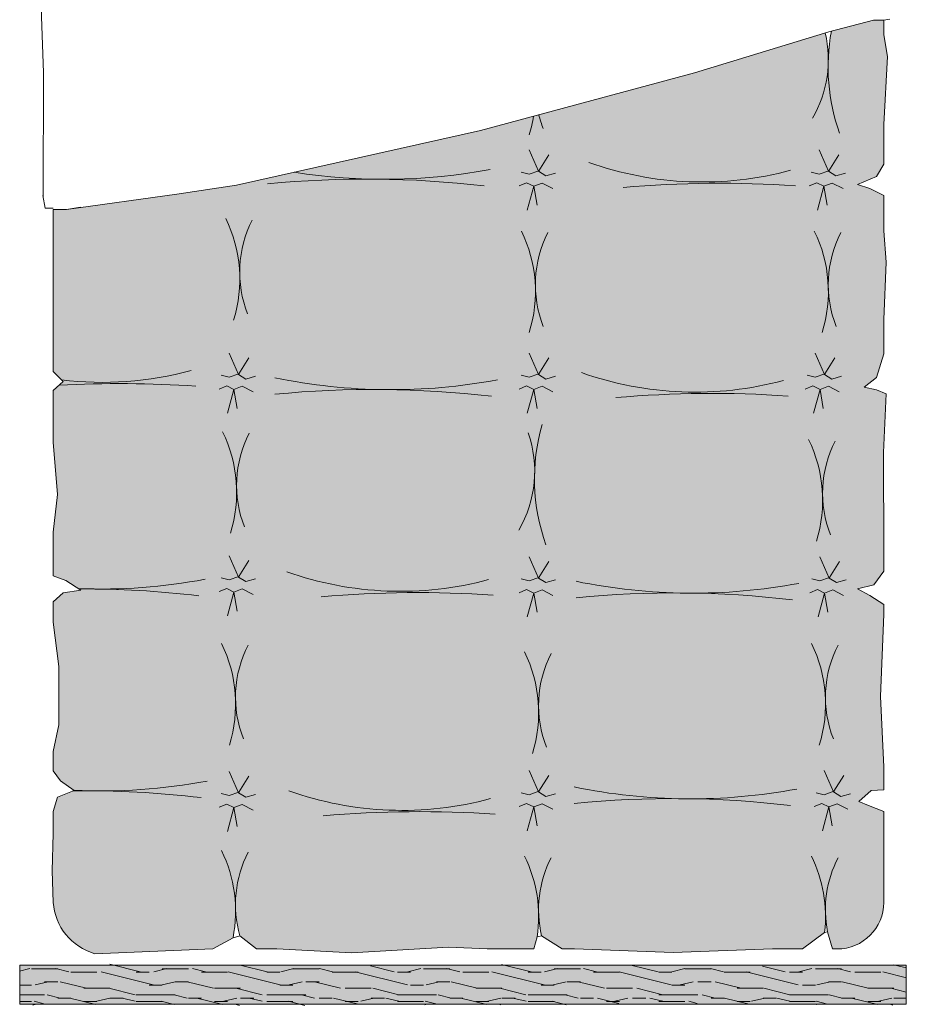
# Model space of a CAD drawing. Units: inches. Extents: x 1994 to 3075, y 3517 to 3950.
# Tile 18 of 58: x 1994.71013 to 1994.74753, y 3553.235 to 3553.27657. Entities that reach past the tile are written whole.
import ezdxf

# ---------------------------------------------------------------- set-up
doc = ezdxf.new("R2010")
doc.units = ezdxf.units.IN
doc.layers.add('A-FURN-REFR', color=8, linetype='Continuous', lineweight=13)
doc.layers.add('A-FURN-REFR-PATT', color=8, linetype='Continuous', lineweight=13)

msp = doc.modelspace()

# ---------------------------------------------------------------- hatches: boundary and pattern name
at = {"layer": 'A-FURN-REFR-PATT'}
h = msp.add_hatch(color=256, dxfattribs=at)
h.set_gradient(color1=(238, 215, 180), color2=(243, 226, 201), one_color=1, tint=0.8700000047683715)
edge = h.paths.add_edge_path()
edge.add_line((1994.745465238979, 3553.252543770607), (1994.745983417828, 3553.25225612802))
edge.add_line((1994.745983417828, 3553.25225612802), (1994.746580376501, 3553.251881311399))
edge.add_line((1994.746580376501, 3553.251881311399), (1994.746580376501, 3553.25147861202))
edge.add_line((1994.746580376501, 3553.25147861202), (1994.746444020425, 3553.247999023068))
edge.add_line((1994.746444020425, 3553.247999023068), (1994.746580376501, 3553.245035426197))
edge.add_line((1994.746580376501, 3553.245035426197), (1994.746580376501, 3553.244057442249))
edge.add_line((1994.746580376501, 3553.244057442249), (1994.746040993021, 3553.244029560099))
edge.add_line((1994.74604099302, 3553.244029560098), (1994.745522814171, 3553.24356933293))
edge.add_line((1994.745522814171, 3553.24356933293), (1994.745925842637, 3553.243396747134))
edge.add_line((1994.745925842637, 3553.243396747134), (1994.746580376501, 3553.243136987305))
edge.add_line((1994.746580376501, 3553.243136987305), (1994.746580376501, 3553.239308473302))
edge.add_ellipse((1994.744611872564, 3553.239308473302), major_axis=(-0.0013954107568795, 0.0013884655449815), ratio=0.9999999999995969, start_angle=134.8570588413608, end_angle=224.8570588413444, ccw=False)
edge.add_line((1994.744611872564, 3553.237339969366), (1994.744419991744, 3553.237339969366))
edge.add_line((1994.744419991744, 3553.237339969366), (1994.744207350188, 3553.238064686622))
edge.add_ellipse((1994.74891501896, 3553.23899557781), major_axis=(-0.0034017353614211, 0.0033848043088335), ratio=0.9999999999961552, start_angle=46.9904168057862, end_angle=56.04239135558288, ccw=False)
edge.add_ellipse((1994.738320716176, 3553.238701604092), major_axis=(0.0040909414474347, 0.0041114046525301), ratio=0.9999999999404371, start_angle=315.9964899997492, end_angle=316.8965310452939)
edge.add_ellipse((1994.74891501896, 3553.23899557781), major_axis=(-0.0034017353615801, 0.0033848043089917), ratio=0.999999999999969, start_angle=45.90260423888249, end_angle=46.99041680598647)
edge.add_ellipse((1994.738320716176, 3553.238701604092), major_axis=(-0.0041114046547348, 0.0040909414496284), ratio=0.9999999999992981, start_angle=218.3076497279251, end_angle=225.9964899996222, ccw=False)
edge.add_line((1994.744082817506, 3553.238040061614), (1994.743146211789, 3553.237339969366))
edge.add_line((1994.743146211789, 3553.237339969366), (1994.741879553322, 3553.237339969366))
edge.add_line((1994.741879553322, 3553.237339969366), (1994.737692562603, 3553.237183674896))
edge.add_line((1994.737692562603, 3553.237183674896), (1994.733531122905, 3553.237339969366))
edge.add_line((1994.733531122905, 3553.237339969366), (1994.733012944056, 3553.237339969366))
edge.add_line((1994.733012944056, 3553.237339969366), (1994.732142059715, 3553.237890147645))
edge.add_ellipse((1994.736811524591, 3553.238996855125), major_axis=(0.003384804308798, 0.0034017353613854), ratio=0.9999999999991601, start_angle=136.9904168061205, end_angle=148.1906707088415, ccw=False)
edge.add_ellipse((1994.726217221807, 3553.238702881407), major_axis=(-0.0041114046563086, 0.0040909414511943), ratio=0.9999999999589329, start_angle=225.9964899994617, end_angle=226.8965310452883)
edge.add_ellipse((1994.736811524591, 3553.238996855125), major_axis=(-0.0034017353616, 0.0033848043090115), ratio=0.9999999999992102, start_angle=45.90260423888252, end_angle=46.99041680597979)
edge.add_ellipse((1994.726217221807, 3553.238702881407), major_axis=(0.0040909414496365, 0.004111404654743), ratio=0.9999999999998221, start_angle=306.35556291123595, end_angle=315.99648999952274, ccw=False)
edge.add_line((1994.731953444552, 3553.237845444061), (1994.731817558786, 3553.237339969366))
edge.add_line((1994.731817558786, 3553.237339969366), (1994.729846297889, 3553.237339969366))
edge.add_line((1994.729846297889, 3553.237339969366), (1994.728214507854, 3553.237409828841))
edge.add_line((1994.728214507854, 3553.237409828841), (1994.724126656494, 3553.237179715257))
edge.add_line((1994.724126656494, 3553.237179715257), (1994.720979688623, 3553.237339969366))
edge.add_line((1994.720979688623, 3553.237339969366), (1994.720116058622, 3553.237339969366))
edge.add_line((1994.720116058622, 3553.237339969366), (1994.719418569442, 3553.237896439695))
edge.add_ellipse((1994.724028450143, 3553.239229745213), major_axis=(0.0033848043087955, 0.003401735361383), ratio=0.9999999999994543, start_angle=136.9904168061405, end_angle=150.9883963242237, ccw=False)
edge.add_ellipse((1994.713434147359, 3553.238935771494), major_axis=(-0.0041114046562385, 0.0040909414511246), ratio=0.9999999999586175, start_angle=225.9964899994838, end_angle=226.8965310452442)
edge.add_ellipse((1994.724028450143, 3553.239229745213), major_axis=(0.0033848043066325, 0.0034017353592091), ratio=0.9999999999427059, start_angle=135.9026042389893, end_angle=136.9904168059202)
edge.add_ellipse((1994.713434147359, 3553.238935771494), major_axis=(0.0040909414496316, 0.004111404654738), ratio=0.9999999999988398, start_angle=303.6775311936519, end_angle=315.99648999963307, ccw=False)
edge.add_line((1994.719124042928, 3553.237811254448), (1994.718273646114, 3553.237339969366))
edge.add_line((1994.718273646114, 3553.237339969366), (1994.713290858704, 3553.237138047984))
edge.add_ellipse((1994.713981582004, 3553.239489970725), major_axis=(0.0017289677196812, 0.0017376161497567), ratio=0.9999999999998783, start_angle=139.1032804179422, end_angle=208.4903617465707, ccw=False)
edge.add_line((1994.711537057931, 3553.239308473302), (1994.711495025274, 3553.240641762328))
edge.add_line((1994.711495025274, 3553.240641762328), (1994.711537057931, 3553.242218732161))
edge.add_line((1994.711537057931, 3553.242218732161), (1994.711537057931, 3553.243139187105))
edge.add_line((1994.711537057931, 3553.243139187105), (1994.711725327103, 3553.243748298751))
edge.add_line((1994.711725327103, 3553.243748298751), (1994.712371387265, 3553.244017270866))
edge.add_ellipse((1994.712804930991, 3553.201258781263), major_axis=(-0.030311711425235, 0.0301608445512322), ratio=0.9999999999998488, start_angle=314.7424189967481, end_angle=315.43798147785856, ccw=False)
edge.add_ellipse((1994.713561032044, 3553.268365279359), major_axis=(0.017178658539876, 0.0172645875167344), ratio=0.9999999999995717, start_angle=223.2793960877664, end_angle=225.1436524008468)
edge.add_ellipse((1994.712804930991, 3553.201258781263), major_axis=(0.0301608445493612, 0.0303117114233546), ratio=0.9999999999998355, start_angle=43.68062949186479, end_angle=44.7424189967496)
edge.add_ellipse((1994.713561032044, 3553.268365279359), major_axis=(-0.0172645875178435, 0.0171786585409796), ratio=0.99999999999105, start_angle=132.1588264661551, end_angle=133.2793960877638, ccw=False)
edge.add_line((1994.712414498921, 3553.244037152568), (1994.711840477486, 3553.244438640111))
edge.add_line((1994.711840477486, 3553.244438640111), (1994.71153705793, 3553.244865040809))
edge.add_line((1994.711537057931, 3553.244865040809), (1994.711537057931, 3553.24567043896))
edge.add_line((1994.711537057931, 3553.24567043896), (1994.711782902294, 3553.246797306171))
edge.add_line((1994.711782902294, 3553.246797306171), (1994.711782902294, 3553.24927102963))
edge.add_line((1994.711782902294, 3553.24927102963), (1994.711537057931, 3553.251135641442))
edge.add_line((1994.711537057931, 3553.251135641442), (1994.711537057931, 3553.25199856799))
edge.add_line((1994.711537057931, 3553.25199856799), (1994.71195562787, 3553.252377566053))
edge.add_line((1994.71195562787, 3553.252377566053), (1994.712704108549, 3553.252492622845))
edge.add_line((1994.712704108549, 3553.252492622845), (1994.712627747323, 3553.252541176693))
edge.add_ellipse((1994.712711338535, 3553.209780570924), major_axis=(-0.0303117114363433, 0.0301608445622852), ratio=0.999999999993631, start_angle=314.74241899675263, end_angle=314.96906421360694, ccw=False)
edge.add_ellipse((1994.713467439589, 3553.27688706902), major_axis=(0.017178658539876, 0.0172645875167344), ratio=0.9999999999995717, start_angle=223.2793960877664, end_angle=225.1436524008468)
edge.add_ellipse((1994.712711338535, 3553.209780570924), major_axis=(0.0301608445493616, 0.030311711423355), ratio=0.9999999999998095, start_angle=43.68062949186329, end_angle=44.7424189967481)
edge.add_ellipse((1994.713467439589, 3553.27688706902), major_axis=(-0.0172645875254605, 0.0171786585485587), ratio=0.9999999999355926, start_angle=132.8607499557009, end_angle=133.279396087769, ccw=False)
edge.add_line((1994.712619025911, 3553.252546722153), (1994.712070779315, 3553.252895321616))
edge.add_line((1994.712070779315, 3553.252895321616), (1994.71153705793, 3553.25309160873))
edge.add_line((1994.711537057931, 3553.25309160873), (1994.711537057931, 3553.254932519226))
edge.add_line((1994.711537057931, 3553.254932519225), (1994.711725327103, 3553.256519614211))
edge.add_line((1994.711725327103, 3553.256519614212), (1994.711537057931, 3553.258729396401))
edge.add_line((1994.711537057931, 3553.258729396401), (1994.711537057931, 3553.26091547788))
edge.add_line((1994.711537057931, 3553.26091547788), (1994.71195562787, 3553.261294475334))
edge.add_line((1994.71195562787, 3553.261294475334), (1994.71153705793, 3553.261720876032))
edge.add_line((1994.711537057931, 3553.261720876032), (1994.711537057931, 3553.268553942703))
edge.add_line((1994.711537057931, 3553.268553942703), (1994.712094041614, 3553.268553942703))
edge.add_line((1994.712094041614, 3553.268553942703), (1994.71674814572, 3553.269206179745))
edge.add_line((1994.71674814572, 3553.269206179745), (1994.719275959651, 3553.269584475613))
edge.add_line((1994.719275959651, 3553.269584475613), (1994.721704827398, 3553.270129843608))
edge.add_ellipse((1994.725499537882, 3553.294187533932), major_axis=(-0.0172645875167904, 0.0171786585399318), ratio=0.999999999999914, start_angle=125.8934301562025, end_angle=135.1436524012626)
edge.add_ellipse((1994.724743436827, 3553.227081035835), major_axis=(-0.0303117114243903, 0.0301608445503917), ratio=0.9999999999981067, start_angle=-46.31937050837215, end_angle=-45.257581003015)
edge.add_ellipse((1994.725499537882, 3553.294187533932), major_axis=(0.0171786585399121, 0.0172645875167707), ratio=0.9999999999996129, start_angle=215.8934301562025, end_angle=223.2793960873529, ccw=False)
edge.add_line((1994.721704827398, 3553.270129843608), (1994.729568916782, 3553.271895613963))
edge.add_line((1994.729568916782, 3553.271895613963), (1994.738589710934, 3553.274322309254))
edge.add_line((1994.738589710934, 3553.274322309254), (1994.744109518087, 3553.276010668554))
edge.add_ellipse((1994.739263851125, 3553.274892925541), major_axis=(0.0035075950851018, 0.0035251403466364), ratio=0.9999999999978005, start_angle=315.5146379508602, end_angle=327.8461990640952, ccw=False)
edge.add_ellipse((1994.752502542269, 3553.27457735018), major_axis=(-0.005865536420184, 0.0058363425837936), ratio=0.999999999997771, start_angle=42.27583207499214, end_angle=44.70724330108613)
edge.add_ellipse((1994.739263851125, 3553.274892925541), major_axis=(-0.0035251403464673, 0.0035075950849335), ratio=0.9999999999932054, start_angle=221.46843742522, end_angle=225.5146379508603)
edge.add_ellipse((1994.752502542269, 3553.27457735018), major_axis=(0.0058363425838986, 0.0058655364202896), ratio=0.9999999999968727, start_angle=124.36393844595369, end_angle=132.2758320749922, ccw=False)
edge.add_line((1994.744366414854, 3553.276084281811), (1994.746144687441, 3553.276547800884))
edge.add_line((1994.746144687441, 3553.276547800884), (1994.746580376501, 3553.276547800884))
edge.add_line((1994.746580376501, 3553.276547800884), (1994.746580376501, 3553.275937280929))
edge.add_line((1994.746580376501, 3553.275937280929), (1994.746736751779, 3553.275017923455))
edge.add_line((1994.746736751779, 3553.275017923455), (1994.7465803765, 3553.272140403147))
edge.add_line((1994.746580376501, 3553.272140403147), (1994.746580376501, 3553.270472078447))
edge.add_line((1994.746580376501, 3553.270472078447), (1994.746276149182, 3553.269955419744))
edge.add_line((1994.746276149182, 3553.269955419744), (1994.745470093312, 3553.269610249368))
edge.add_line((1994.745470093312, 3553.269610249368), (1994.745988272162, 3553.269437663573))
edge.add_line((1994.745988272162, 3553.269437663573), (1994.7465803765, 3553.269148924124))
edge.add_line((1994.746580376501, 3553.269148924124), (1994.746580376501, 3553.267653184612))
edge.add_line((1994.746580376501, 3553.267653184612), (1994.746679176587, 3553.266331127757))
edge.add_line((1994.746679176587, 3553.266331127757), (1994.7465803765, 3553.263913835225))
edge.add_line((1994.746580376501, 3553.263913835225), (1994.746580376501, 3553.262466545988))
edge.add_line((1994.746580376501, 3553.262466545988), (1994.746271294849, 3553.261460679889))
edge.add_line((1994.746271294849, 3553.261460679889), (1994.745753115999, 3553.261057981117))
edge.add_line((1994.745753115999, 3553.261057981117), (1994.746271294849, 3553.260942923717))
edge.add_line((1994.746271294849, 3553.260942923717), (1994.746674322254, 3553.260770338529))
edge.add_line((1994.746674322254, 3553.260770338529), (1994.74655917187, 3553.258296615677))
edge.add_line((1994.74655917187, 3553.258296615677), (1994.746580376501, 3553.25406739227))
edge.add_line((1994.746580376501, 3553.25406739227), (1994.746580376501, 3553.253291640363))
edge.add_line((1994.746580376501, 3553.253291640363), (1994.746156143405, 3553.252716355795))
edge.add_line((1994.746156143405, 3553.252716355795), (1994.745465238979, 3553.252543770607))
edge = h.paths.add_edge_path(flags=16)
edge.add_ellipse((1994.737756386553, 3553.209608254897), major_axis=(0.030160844549362, 0.0303117114233554), ratio=0.9999999999997834, start_angle=43.68062949186179, end_angle=44.74241899674661)
edge.add_ellipse((1994.738512487607, 3553.276714752993), major_axis=(0.0171786585398764, 0.0172645875167348), ratio=0.9999999999995255, start_angle=223.2793960877637, end_angle=225.1436524008441)
edge = h.paths.add_edge_path(flags=16)
edge.add_ellipse((1994.72687704885, 3553.257511810059), major_axis=(-0.0035251403466965, 0.0035075950851616), ratio=0.9999999999998879, start_angle=221.4684374256727, end_angle=225.514637950396)
edge.add_ellipse((1994.740115739994, 3553.257196234698), major_axis=(0.0058363425840069, 0.0058655364203984), ratio=0.9999999999987389, start_angle=132.2758320752676, end_angle=134.7072433008111)
h.paths.add_polyline_path([(1994.732021808397, 3553.253023267114), (1994.731986786092, 3553.253010769348), (1994.73200619594, 3553.252998522719)], flags=16)
edge = h.paths.add_edge_path(flags=16)
edge.add_ellipse((1994.726217221807, 3553.247322021218), major_axis=(0.0040909414477731, 0.0041114046528702), ratio=0.9999999999458513, start_angle=315.9964899995724, end_angle=316.8965310452884)
edge.add_ellipse((1994.736811524591, 3553.247615994937), major_axis=(-0.0034017353615801, 0.0033848043089917), ratio=0.999999999999969, start_angle=45.90260423888249, end_angle=46.99041680598647)
h.paths.add_polyline_path([(1994.73200619594, 3553.261594210102), (1994.732021808397, 3553.261618954497), (1994.731986786092, 3553.261606456731)], flags=16)
edge = h.paths.add_edge_path(flags=16)
edge.add_ellipse((1994.748793777434, 3553.256584102472), major_axis=(-0.0034017353616, 0.0033848043090115), ratio=0.9999999999992102, start_angle=45.90260423888252, end_angle=46.99041680597979)
edge.add_ellipse((1994.73819947465, 3553.256290128754), major_axis=(0.0040909414477996, 0.0041114046528968), ratio=0.9999999999466499, start_angle=315.996489999578, end_angle=316.8965310452884)
h.paths.add_polyline_path([(1994.744250725601, 3553.253010769348), (1994.744270135448, 3553.252998522719), (1994.744285747906, 3553.253023267114)], flags=16)
edge = h.paths.add_edge_path(flags=16)
edge.add_ellipse((1994.725807702035, 3553.285306483294), major_axis=(0.0171786585398506, 0.0172645875167089), ratio=0.9999999999995244, start_angle=223.279396087769, end_angle=225.1436524008441)
edge.add_ellipse((1994.725051600982, 3553.218199985198), major_axis=(0.0301608445493262, 0.0303117114233194), ratio=0.9999999999998141, start_angle=43.68062949186629, end_angle=44.74241899674811)
edge = h.paths.add_edge_path(flags=16)
edge.add_ellipse((1994.74891501896, 3553.247973753577), major_axis=(-0.0034017353616, 0.0033848043090115), ratio=0.9999999999992102, start_angle=45.90260423888252, end_angle=46.99041680597979)
edge.add_ellipse((1994.738320716176, 3553.247679779859), major_axis=(0.0040909414477996, 0.0041114046528968), ratio=0.9999999999466499, start_angle=315.996489999578, end_angle=316.8965310452884)
edge = h.paths.add_edge_path(flags=16)
edge.add_ellipse((1994.726082432568, 3553.265091023611), major_axis=(0.0040909414477996, 0.0041114046528968), ratio=0.9999999999466499, start_angle=315.996489999578, end_angle=316.8965310452884)
edge.add_ellipse((1994.736676735351, 3553.26538499733), major_axis=(-0.0034017353616, 0.0033848043090115), ratio=0.9999999999992102, start_angle=45.90260423888252, end_angle=46.99041680597979)
h.paths.add_polyline_path([(1994.74405918212, 3553.261606456731), (1994.744078591968, 3553.261594210102), (1994.744094204425, 3553.261618954497)], flags=16)
edge = h.paths.add_edge_path(flags=16)
edge.add_ellipse((1994.749034005182, 3553.26538499733), major_axis=(-0.0034017353615801, 0.0033848043089917), ratio=0.999999999999969, start_angle=45.90260423888249, end_angle=46.99041680598647)
edge.add_ellipse((1994.738439702398, 3553.265091023611), major_axis=(0.0040909414477724, 0.0041114046528695), ratio=0.9999999999457356, start_angle=315.9964899995779, end_angle=316.896531045294)
h.paths.add_polyline_path([(1994.732021808397, 3553.243996435937), (1994.731986786092, 3553.24398393817), (1994.73200619594, 3553.243971691542)], flags=16)
edge = h.paths.add_edge_path(flags=16)
edge.add_ellipse((1994.737679105019, 3553.20092495741), major_axis=(0.0301608445494179, 0.0303117114234116), ratio=0.9999999999999388, start_angle=43.68062949186479, end_angle=44.74241899675109)
edge.add_ellipse((1994.738435206073, 3553.268031455506), major_axis=(0.0171786585398771, 0.0172645875167355), ratio=0.9999999999995772, start_angle=223.2793960877664, end_angle=225.1436524008493)
h.paths.add_polyline_path([(1994.744468735191, 3553.243996435937), (1994.744433712885, 3553.24398393817), (1994.744453122734, 3553.243971691542)], flags=16)
h.paths.add_polyline_path([(1994.73200619594, 3553.270171481), (1994.732021808397, 3553.270196225395), (1994.731986786092, 3553.270183727629)], flags=16)
h.paths.add_polyline_path([(1994.719369026331, 3553.253065718053), (1994.719334004026, 3553.253053220288), (1994.719353413874, 3553.253040973658)], flags=16)
edge = h.paths.add_edge_path(flags=16)
edge.add_ellipse((1994.713477879544, 3553.256619851287), major_axis=(-0.0041114046560738, 0.0040909414509607), ratio=0.999999999962278, start_angle=225.9964899995778, end_angle=226.8965310452884)
edge.add_ellipse((1994.724072182329, 3553.256913825005), major_axis=(0.0033848043069108, 0.0034017353594889), ratio=0.9999999999478042, start_angle=135.9026042388825, end_angle=136.9904168059803)
h.paths.add_polyline_path([(1994.744223325676, 3553.270183727629), (1994.744242735524, 3553.270171481), (1994.744258347981, 3553.270196225395)], flags=16)
edge = h.paths.add_edge_path(flags=16)
edge.add_ellipse((1994.713434147359, 3553.247679779859), major_axis=(0.004090941447773, 0.0041114046528701), ratio=0.999999999945836, start_angle=315.9964899995722, end_angle=316.896531045288)
edge.add_ellipse((1994.724028450143, 3553.247973753577), major_axis=(-0.0034017353616392, 0.0033848043090505), ratio=0.999999999998303, start_angle=45.9026042388825, end_angle=46.99041680598649)
h.paths.add_polyline_path([(1994.719353413874, 3553.261594210102), (1994.719369026331, 3553.261618954497), (1994.719334004026, 3553.261606456731)], flags=16)
edge = h.paths.add_edge_path(flags=16)
edge.add_ellipse((1994.713610336299, 3553.265618953796), major_axis=(-0.0041114046594229, 0.0040909414542932), ratio=0.9999999998956695, start_angle=225.9964899995777, end_angle=226.896531045288)
edge.add_ellipse((1994.724204639084, 3553.265912927514), major_axis=(-0.0034017353616, 0.0033848043090115), ratio=0.9999999999992102, start_angle=45.90260423888252, end_angle=46.99041680597979)
h.paths.add_polyline_path([(1994.719369026331, 3553.243962374809), (1994.719334004026, 3553.243949877043), (1994.719353413874, 3553.243937630414)], flags=16)
msp.add_hatch(color=256, dxfattribs=at).paths.add_polyline_path([(1994.74752711248, 3553.236652102432), (1994.710125537677, 3553.236652102432), (1994.710125537677, 3553.235003554395), (1994.74752711248, 3553.235003554395)])
h = msp.add_hatch(dxfattribs=at)
h.set_pattern_fill('LEGNO1', color=256, scale=0.005511811023622, style=0, pattern_type=2)
h.set_pattern_definition([(0, (2000.356371596277, 3548.843453761226), (0, 0.005511811023622), [0.0011023622047244, -0.0016535433070866, 0.0005511811023622, -0.0022047244094488]), (0, (2000.360229863994, 3548.843591556501), (0, 0.005511811023622), [0.0011023622047244, -0.0044094488188976]), (0, (2000.359678682892, 3548.843867147053), (0, 0.005511811023622), [0.0005511811023622, -0.0049606299212598]), (0, (2000.356647186829, 3548.844004942328), (0, 0.005511811023622), [0.0002755905511811, -0.0038582677165354, 0.0002755905511811, -0.0011023622047244]), (0, (2000.358576320687, 3548.844280532879), (0, 0.005511811023622), [0.0011023622047244, -0.0016535433070866, 0.0002755905511811, -0.0024803149606299]), (0, (2000.357198367931, 3548.844418328155), (0, 0.005511811023622), [0.0008267716535433, -0.0046850393700787]), (0, (2000.358576320687, 3548.844556123431), (0, 0.005511811023622), [0.0016535433070866, -0.0038582677165354]), (0, (2000.356922777379, 3548.844693918706), (0, 0.005511811023622), [0.0011023622047244, -0.0044094488188976]), (0, (2000.35912750179, 3548.844831713982), (0, 0.005511811023622), [0.002755905511811, -0.002755905511811]), (0, (2000.357473958482, 3548.845107304533), (0, 0.005511811023622), [0.0005511811023622, -0.0016535433070866, 0.0011023622047244, -0.0022047244094488]), (0, (2000.361332226199, 3548.845245099808), (0, 0.005511811023622), [0.0011023622047244, -0.0044094488188976]), (0, (2000.360229863994, 3548.845382895084), (0, 0.005511811023622), [0.0005511811023622, -0.0049606299212598]), (0, (2000.35912750179, 3548.84552069036), (0, 0.005511811023622), [0.0005511811023622, -0.0049606299212598]), (0, (2000.356371596277, 3548.845658485635), (0, 0.005511811023622), [0.0011023622047244, -0.0044094488188976]), (0, (2000.35912750179, 3548.845796280911), (0, 0.005511811023622), [0.0011023622047244, -0.0044094488188976]), (0, (2000.35912750179, 3548.846071871462), (0, 0.005511811023622), [0.0011023622047244, -0.0011023622047244, 0.0011023622047244, -0.0022047244094488]), (0, (2000.358025139584, 3548.846347462013), (0, 0.005511811023622), [0.0005511811023622, -0.002755905511811, 0.0011023622047244, -0.0011023622047244]), (0, (2000.35912750179, 3548.846485257289), (0, 0.005511811023622), [0.0016535433070866, -0.0038582677165354]), (0, (2000.35912750179, 3548.84676084784), (0, 0.005511811023622), [0.0011023622047244, -0.0044094488188976]), (0, (2000.356922777379, 3548.846898643116), (0, 0.005511811023622), [0.0016535433070866, -0.0022047244094488, 0.0005511811023622, -0.0011023622047244]), (0, (2000.356922777379, 3548.847174233667), (0, 0.005511811023622), [0.002755905511811, -0.002755905511811]), (0, (2000.360229863994, 3548.847312028942), (0, 0.005511811023622), [0.0005511811023622, -0.0049606299212598]), (0, (2000.358576320687, 3548.847449824219), (0, 0.005511811023622), [0.0011023622047244, -0.0044094488188976]), (0, (2000.357473958482, 3548.847587619493), (0, 0.005511811023622), [0.0005511811023622, -0.0022047244094488, 0.0005511811023622, -0.0022047244094488]), (0, (2000.356922777379, 3548.84772541477), (0, 0.005511811023622), [0.0005511811023622, -0.0016535433070866, 0.0011023622047244, -0.0022047244094488]), (0, (2000.358025139584, 3548.847863210045), (0, 0.005511811023622), [0.0005511811023622, -0.002755905511811, 0.0005511811023622, -0.0016535433070866]), (0, (2000.35912750179, 3548.84800100532), (0, 0.005511811023622), [0.0016535433070866, -0.0038582677165354]), (0, (2000.356922777379, 3548.848276595871), (0, 0.005511811023622), [0.0011023622047244, -0.0044094488188976]), (0, (2000.359678682892, 3548.848414391147), (0, 0.005511811023622), [0.0005511811023622, -0.0049606299212598]), (0, (2000.360781045096, 3548.848552186423), (0, 0.005511811023622), [0.0005511811023622, -0.0049606299212598]), (14.03624347, (2000.360229863994, 3548.843867147053), (0.0055118110234648, -2.016e-13), [0.0005677165354331, -0.0221580619543307]), (14.03624347, (2000.360781045096, 3548.845107304533), (0.0055118110234648, -2.016e-13), [0.0005677165354331, -0.0221580619543307]), (14.03624347, (2000.360229863994, 3548.848414391147), (0.0055118110234648, -2.016e-13), [0.0005677165354331, -0.0221580619543307]), (14.03624347, (2000.358576320687, 3548.846347462013), (0.0055118110234648, -2.016e-13), [0.0005677165354331, -0.0221580619543307]), (14.03624347, (2000.359678682892, 3548.847174233667), (0.0055118110234648, -2.016e-13), [0.0005677165354331, -0.0221580619543307]), (14.03624347, (2000.360229863994, 3548.84676084784), (0.0055118110234648, -2.016e-13), [0.0005677165354331, -0.0221580619543307]), (14.03624347, (2000.357473958482, 3548.84772541477), (0.0055118110234648, -2.016e-13), [0.0005677165354331, -0.0221580619543307]), (14.03624347, (2000.359678682892, 3548.847449824219), (0.0055118110234648, -2.016e-13), [0.0005677165354331, -0.0221580619543307]), (14.03624347, (2000.360781045096, 3548.845382895084), (0.0055118110234648, -2.016e-13), [0.0011354330708661, -0.0215903454188977]), (14.03624347, (2000.360229863994, 3548.845796280911), (0.0055118110234648, -2.016e-13), [0.0011354330708661, -0.0215903454188977]), (14.03624347, (2000.360229863994, 3548.846071871462), (0.0055118110234648, -2.016e-13), [0.0011354330708661, -0.0215903454188977]), (165.96375653, (2000.358576320687, 3548.844280532879), (-0.0055118110234648, -2.016e-13), [0.0005677165354331, -0.0011354330708661, 0.0005677165354331, -0.0204549123480315]), (165.96375653, (2000.357473958482, 3548.845107304533), (-0.0055118110234648, -2.016e-13), [0.0005677165354331, -0.0221580619543307]), (165.96375653, (2000.357473958482, 3548.847587619493), (-0.0055118110234648, -2.016e-13), [0.0011354330708661, -0.0215903454188977]), (194.03624347, (2000.360229863994, 3548.843591556501), (-0.0055118110234648, 2.016e-13), [0.0005677165354331, -0.0221580619543307]), (345.96375653, (2000.361332226199, 3548.843591556501), (0.0055118110234648, 2.016e-13), [0.0005677165354331, -0.0221580619543307]), (345.96375653, (2000.359678682892, 3548.84552069036), (0.0055118110234648, 2.016e-13), [0.0005677165354331, -0.0221580619543307]), (345.96375653, (2000.360781045096, 3548.846485257289), (0.0055118110234648, 2.016e-13), [0.0005677165354331, -0.0221580619543307]), (345.96375653, (2000.358576320687, 3548.846898643116), (0.0055118110234648, 2.016e-13), [0.0005677165354331, -0.0221580619543307]), (345.96375653, (2000.358025139584, 3548.847587619493), (0.0055118110234648, 2.016e-13), [0.0005677165354331, -0.0221580619543307]), (345.96375653, (2000.358576320687, 3548.847863210045), (0.0055118110234648, 2.016e-13), [0.0005677165354331, -0.0221580619543307]), (345.96375653, (2000.358576320687, 3548.846898643116), (0.0055118110234648, 2.016e-13), [0.0005677165354331, -0.0221580619543307]), (345.96375653, (2000.360229863994, 3548.84772541477), (0.0055118110234648, 2.016e-13), [0.0022708661417323, -0.0204549123480315]), (345.96375653, (2000.356922777379, 3548.844004942328), (0.0055118110234648, 2.016e-13), [0.0022708661417323, -0.0204549123480315]), (345.96375653, (2000.357473958482, 3548.844418328155), (0.0055118110234648, 2.016e-13), [0.0022708661417323, -0.0204549123480315]), (345.96375653, (2000.358025139584, 3548.844693918706), (0.0055118110234648, 2.016e-13), [0.0005677165354331, -0.0011354330708661, 0.0011354330708661, -0.0198871958125984]), (345.96375653, (2000.358025139584, 3548.845107304533), (0.0055118110234648, 2.016e-13), [0.0011354330708661, -0.0011354330708661, 0.0011354330708661, -0.0193194792771654]), (345.96375653, (2000.357473958482, 3548.845658485635), (0.0055118110234648, 2.016e-13), [0.0022708661417323, -0.0204549123480315]), (345.96375653, (2000.356922777379, 3548.846071871462), (0.0055118110234648, 2.016e-13), [0.0022708661417323, -0.0204549123480315]), (345.96375653, (2000.356922777379, 3548.846347462013), (0.0055118110234648, 2.016e-13), [0.0022708661417323, -0.0204549123480315]), (345.96375653, (2000.360781045096, 3548.84800100532), (0.0055118110234648, 2.016e-13), [0.0005677165354331, -0.0221580619543307]), (345.9637675300001, (2000.361332226199, 3548.848552186423), (0.0055118110234647, 1.0583933e-09), [0.0011354330708661, -0.0215903454188977]), (345.9637675300001, (2000.358025139584, 3548.848276595871), (0.0055118110234647, 1.0583933e-09), [0.0011354330708661, -0.0215903454188977]), (345.96375753, (2000.357473958482, 3548.843453761226), (0.0055118110234648, 9.64008e-11), [0.0022708661417323, -0.0204549123480315]), (345.96375753, (2000.360781045096, 3548.847312028942), (0.0055118110234648, 9.64008e-11), [0.0017031496062992, -0.0210226288834646]), (345.96375753, (2000.361332226199, 3548.846898643116), (0.0055118110234648, 9.64008e-11), [0.0034062992125984, -0.0193194792771654])])
h.paths.add_polyline_path([(1994.74752711248, 3553.236652102432), (1994.710125537677, 3553.236652102432), (1994.710125537677, 3553.235003554395), (1994.74752711248, 3553.235003554395)])

# ---------------------------------------------------------------- linework, layer by layer
at = {"layer": 'A-FURN-REFR'}
for p, q in [((1994.710937653731, 3553.279644278879), (1994.711129775177, 3553.274346052923)), ((1994.74425661957, 3553.276055662909), (1994.746144687441, 3553.276547800884)), ((1994.746144687441, 3553.276547800884), (1994.746580376501, 3553.276547800884)), ((1994.746580376501, 3553.276547800884), (1994.746826688549, 3553.27659207166)), ((1994.746580376501, 3553.276547800884), (1994.746580376501, 3553.275937280929)), ((1994.738589710934, 3553.274322309254), (1994.74425661957, 3553.276055662909)), ((1994.746736751779, 3553.275017923455), (1994.746580376501, 3553.275937280929)), ((1994.746580376501, 3553.272140403147), (1994.746736751779, 3553.275017923455)), ((1994.711129775177, 3553.274346052923), (1994.711113967212, 3553.269074274324)), ((1994.729568916782, 3553.271895613963), (1994.738589710934, 3553.274322309254)), ((1994.719275959651, 3553.269584475613), (1994.729568916782, 3553.271895613963)), ((1994.746580376501, 3553.272140403147), (1994.746580376501, 3553.270472078447)), ((1994.73200619594, 3553.270171481), (1994.731612882744, 3553.27107177963)), ((1994.744242735524, 3553.270171481), (1994.743849422327, 3553.27107177963)), ((1994.732021808397, 3553.270196225395), (1994.732445338485, 3553.270867483972)), ((1994.744258347981, 3553.270196225395), (1994.744681878069, 3553.270867483972)), ((1994.731612882744, 3553.270050299618), (1994.732021808397, 3553.270196225395)), ((1994.732313897828, 3553.269977336729), (1994.73200619594, 3553.270171481)), ((1994.743849422327, 3553.270050299618), (1994.744258347981, 3553.270196225395)), ((1994.744550437411, 3553.269977336729), (1994.744242735524, 3553.270171481)), ((1994.746276149182, 3553.269955419744), (1994.746580376501, 3553.270472078447)), ((1994.731276980012, 3553.270137855084), (1994.731612882744, 3553.270050299618)), ((1994.732722823482, 3553.270094077351), (1994.732313897828, 3553.269977336729)), ((1994.743513519595, 3553.270137855084), (1994.743849422327, 3553.270050299618)), ((1994.744959363065, 3553.270094077351), (1994.744550437411, 3553.269977336729)), ((1994.745470093312, 3553.269610249368), (1994.746276149182, 3553.269955419744)), ((1994.71674814572, 3553.269206179745), (1994.719275959651, 3553.269584475613)), ((1994.731189353408, 3553.269554152405), (1994.731510651707, 3553.269685485605)), ((1994.731510651707, 3553.269685485605), (1994.731817345571, 3553.269539559828)), ((1994.731817345571, 3553.269539559828), (1994.731539860574, 3553.268532672393)), ((1994.732167853489, 3553.269670893028), (1994.731817345571, 3553.269539559828)), ((1994.731817345571, 3553.269539559828), (1994.731948786228, 3553.268736968482)), ((1994.732620591692, 3553.269437411783), (1994.732167853489, 3553.269670893028)), ((1994.743425892991, 3553.269554152405), (1994.74374719129, 3553.269685485605)), ((1994.74374719129, 3553.269685485605), (1994.744053885154, 3553.269539559828)), ((1994.744053885154, 3553.269539559828), (1994.743776400158, 3553.268532672393)), ((1994.744404393072, 3553.269670893028), (1994.744053885154, 3553.269539559828)), ((1994.744053885154, 3553.269539559828), (1994.744185325811, 3553.268736968482)), ((1994.744857131275, 3553.269437411783), (1994.744404393072, 3553.269670893028)), ((1994.745988272162, 3553.269437663573), (1994.745470093312, 3553.269610249368)), ((1994.746580376501, 3553.269148924124), (1994.745988272162, 3553.269437663573)), ((1994.711098697876, 3553.269150558865), (1994.711206060319, 3553.268614183581)), ((1994.712094041614, 3553.268553942703), (1994.71674814572, 3553.269206179745)), ((1994.746580376501, 3553.269148924124), (1994.746580376501, 3553.267653184612)), ((1994.711206060319, 3553.268614183581), (1994.711537057931, 3553.268614183581)), ((1994.712094041614, 3553.268553942703), (1994.711537057931, 3553.268553942703)), ((1994.711537057931, 3553.261720876032), (1994.711537057931, 3553.268553942703)), ((1994.712094041614, 3553.268553942703), (1994.712683841166, 3553.2686600201)), ((1994.746679176587, 3553.266331127757), (1994.746580376501, 3553.267653184612)), ((1994.746580376501, 3553.263913835225), (1994.746679176587, 3553.266331127757)), ((1994.746580376501, 3553.263913835225), (1994.746580376501, 3553.262466545988)), ((1994.719353413874, 3553.261594210102), (1994.718960100677, 3553.262494508731)), ((1994.719369026331, 3553.261618954497), (1994.719792556418, 3553.262290213074)), ((1994.73200619594, 3553.261594210102), (1994.731612882744, 3553.262494508731)), ((1994.732021808397, 3553.261618954497), (1994.732445338485, 3553.262290213074)), ((1994.744078591968, 3553.261594210102), (1994.743685278772, 3553.262494508731)), ((1994.744094204425, 3553.261618954497), (1994.744517734513, 3553.262290213074)), ((1994.746271294849, 3553.261460679889), (1994.746580376501, 3553.262466545988)), ((1994.711537057931, 3553.261720876032), (1994.71195562787, 3553.261294475334)), ((1994.718624197945, 3553.261560584186), (1994.718960100677, 3553.26147302872)), ((1994.718960100677, 3553.26147302872), (1994.719369026331, 3553.261618954497)), ((1994.719661115761, 3553.261400065832), (1994.719353413874, 3553.261594210102)), ((1994.720070041415, 3553.261516806453), (1994.719661115761, 3553.261400065832)), ((1994.731276980012, 3553.261560584186), (1994.731612882744, 3553.26147302872)), ((1994.731612882744, 3553.26147302872), (1994.732021808397, 3553.261618954497)), ((1994.732313897828, 3553.261400065832), (1994.73200619594, 3553.261594210102)), ((1994.732722823482, 3553.261516806453), (1994.732313897828, 3553.261400065832)), ((1994.743349376039, 3553.261560584186), (1994.743685278772, 3553.26147302872)), ((1994.743685278772, 3553.26147302872), (1994.744094204425, 3553.261618954497)), ((1994.744386293856, 3553.261400065832), (1994.744078591968, 3553.261594210102)), ((1994.744795219509, 3553.261516806453), (1994.744386293856, 3553.261400065832)), ((1994.745753115999, 3553.261057981117), (1994.746271294849, 3553.261460679889)), ((1994.71195562787, 3553.261294475334), (1994.711537057931, 3553.26091547788)), ((1994.718536571342, 3553.260976881507), (1994.71885786964, 3553.261108214707)), ((1994.71885786964, 3553.261108214707), (1994.719164563504, 3553.26096228893)), ((1994.719515071422, 3553.261093622129), (1994.719164563504, 3553.26096228893)), ((1994.719967809625, 3553.260860140885), (1994.719515071422, 3553.261093622129)), ((1994.731189353408, 3553.260976881507), (1994.731510651707, 3553.261108214707)), ((1994.731510651707, 3553.261108214707), (1994.731817345571, 3553.26096228893)), ((1994.732167853489, 3553.261093622129), (1994.731817345571, 3553.26096228893)), ((1994.732620591692, 3553.260860140885), (1994.732167853489, 3553.261093622129)), ((1994.743261749436, 3553.260976881507), (1994.743583047734, 3553.261108214707)), ((1994.743583047734, 3553.261108214707), (1994.743889741599, 3553.26096228893)), ((1994.744240249517, 3553.261093622129), (1994.743889741599, 3553.26096228893)), ((1994.74469298772, 3553.260860140885), (1994.744240249517, 3553.261093622129)), ((1994.746271294849, 3553.260942923717), (1994.745753115999, 3553.261057981117)), ((1994.711537057931, 3553.258729396401), (1994.711537057931, 3553.26091547788)), ((1994.719164563504, 3553.26096228893), (1994.718887078508, 3553.259955401496)), ((1994.719164563504, 3553.26096228893), (1994.719296004161, 3553.260159697585)), ((1994.731817345571, 3553.26096228893), (1994.731539860574, 3553.259955401496)), ((1994.731817345571, 3553.26096228893), (1994.731948786228, 3553.260159697585)), ((1994.743889741599, 3553.26096228893), (1994.743612256602, 3553.259955401496)), ((1994.743889741599, 3553.26096228893), (1994.744021182256, 3553.260159697585)), ((1994.746674322254, 3553.260770338529), (1994.746271294849, 3553.260942923717)), ((1994.74655917187, 3553.258296615677), (1994.746674322254, 3553.260770338529)), ((1994.711537057931, 3553.258729396401), (1994.711725327103, 3553.256519614212)), ((1994.746580376501, 3553.25406739227), (1994.74655917187, 3553.258296615677)), ((1994.711725327103, 3553.256519614212), (1994.711537057931, 3553.254932519225)), ((1994.711537057931, 3553.25309160873), (1994.711537057931, 3553.254932519225)), ((1994.719353413874, 3553.253040973658), (1994.718960100677, 3553.253941272288)), ((1994.746580376501, 3553.25406739227), (1994.746580376501, 3553.253291640363)), ((1994.719369026331, 3553.253065718053), (1994.719792556418, 3553.25373697663)), ((1994.73200619594, 3553.252998522719), (1994.731612882744, 3553.253898821348)), ((1994.732021808397, 3553.253023267114), (1994.732445338485, 3553.25369452569)), ((1994.744270135448, 3553.252998522719), (1994.743876822252, 3553.253898821348)), ((1994.744285747906, 3553.253023267114), (1994.744709277993, 3553.25369452569)), ((1994.746156143405, 3553.252716355795), (1994.746580376501, 3553.253291640363)), ((1994.711537057931, 3553.25309160873), (1994.712070779315, 3553.252895321616)), ((1994.712070779315, 3553.252895321616), (1994.712704108549, 3553.252492622845)), ((1994.718624197945, 3553.253007347742), (1994.718960100677, 3553.252919792276)), ((1994.718960100677, 3553.252919792276), (1994.719369026331, 3553.253065718053)), ((1994.719661115761, 3553.252846829387), (1994.719353413874, 3553.253040973658)), ((1994.720070041415, 3553.252963570009), (1994.719661115761, 3553.252846829387)), ((1994.731276980012, 3553.252964896802), (1994.731612882744, 3553.252877341336)), ((1994.731612882744, 3553.252877341336), (1994.732021808397, 3553.253023267114)), ((1994.732313897828, 3553.252804378447), (1994.73200619594, 3553.252998522719)), ((1994.732722823482, 3553.25292111907), (1994.732313897828, 3553.252804378447)), ((1994.74354091952, 3553.252964896802), (1994.743876822252, 3553.252877341336)), ((1994.743876822252, 3553.252877341336), (1994.744285747906, 3553.253023267114)), ((1994.744577837336, 3553.252804378447), (1994.744270135448, 3553.252998522719)), ((1994.74498676299, 3553.25292111907), (1994.744577837336, 3553.252804378447)), ((1994.745465238979, 3553.252543770607), (1994.746156143405, 3553.252716355795)), ((1994.71195562787, 3553.252377566053), (1994.711537057931, 3553.25199856799)), ((1994.712704108549, 3553.252492622845), (1994.71195562787, 3553.252377566053)), ((1994.718536571342, 3553.252423645063), (1994.71885786964, 3553.252554978263)), ((1994.71885786964, 3553.252554978263), (1994.719164563504, 3553.252409052485)), ((1994.719164563504, 3553.252409052485), (1994.718887078508, 3553.251402165051)), ((1994.719515071422, 3553.252540385685), (1994.719164563504, 3553.252409052485)), ((1994.719164563504, 3553.252409052485), (1994.719296004161, 3553.251606461139)), ((1994.719967809625, 3553.252306904441), (1994.719515071422, 3553.252540385685)), ((1994.731189353408, 3553.252381194124), (1994.731510651707, 3553.252512527323)), ((1994.731510651707, 3553.252512527323), (1994.731817345571, 3553.252366601546)), ((1994.731817345571, 3553.252366601546), (1994.731539860574, 3553.251359714112)), ((1994.732167853489, 3553.252497934746), (1994.731817345571, 3553.252366601546)), ((1994.731817345571, 3553.252366601546), (1994.731948786228, 3553.251564010201)), ((1994.732620591692, 3553.252264453501), (1994.732167853489, 3553.252497934746)), ((1994.743453292917, 3553.252381194124), (1994.743774591215, 3553.252512527323)), ((1994.743774591215, 3553.252512527323), (1994.744081285079, 3553.252366601546)), ((1994.744081285079, 3553.252366601546), (1994.743803800082, 3553.251359714112)), ((1994.744431792997, 3553.252497934746), (1994.744081285079, 3553.252366601546)), ((1994.744081285079, 3553.252366601546), (1994.744212725736, 3553.251564010201)), ((1994.7448845312, 3553.252264453501), (1994.744431792997, 3553.252497934746)), ((1994.745983417828, 3553.25225612802), (1994.745465238979, 3553.252543770607)), ((1994.711537057931, 3553.251135641442), (1994.711537057931, 3553.25199856799)), ((1994.746580376501, 3553.251881311399), (1994.745983417828, 3553.25225612802)), ((1994.746580376501, 3553.251881311399), (1994.746580376501, 3553.25147861202)), ((1994.746444020425, 3553.247999023068), (1994.746580376501, 3553.25147861202)), ((1994.711537057931, 3553.251135641442), (1994.711782902294, 3553.24927102963)), ((1994.711782902294, 3553.24927102963), (1994.711782902294, 3553.246797306171)), ((1994.746580376501, 3553.245035426197), (1994.746444020425, 3553.247999023068)), ((1994.711782902294, 3553.246797306171), (1994.711537057931, 3553.24567043896)), ((1994.711537057931, 3553.244865040809), (1994.711537057931, 3553.24567043896)), ((1994.711537057931, 3553.244865040809), (1994.711840477486, 3553.244438640111)), ((1994.719353413874, 3553.243937630414), (1994.718960100677, 3553.244837929043)), ((1994.73200619594, 3553.243971691542), (1994.731612882744, 3553.24487199017)), ((1994.744453122734, 3553.243971691542), (1994.744059809537, 3553.24487199017)), ((1994.746580376501, 3553.245035426197), (1994.746580376501, 3553.244057442249)), ((1994.711840477486, 3553.244438640111), (1994.712416231528, 3553.244035940731)), ((1994.719369026331, 3553.243962374809), (1994.719792556418, 3553.244633633386)), ((1994.732021808397, 3553.243996435937), (1994.732445338485, 3553.244667694513)), ((1994.744468735191, 3553.243996435937), (1994.744892265278, 3553.244667694513)), ((1994.712416231528, 3553.244035940731), (1994.711725327103, 3553.243748298751)), ((1994.718960100677, 3553.243816449032), (1994.719369026331, 3553.243962374809)), ((1994.731612882744, 3553.243850510158), (1994.732021808397, 3553.243996435937)), ((1994.732313897828, 3553.243777547269), (1994.73200619594, 3553.243971691542)), ((1994.744059809537, 3553.243850510158), (1994.744468735191, 3553.243996435937)), ((1994.744760824621, 3553.243777547269), (1994.744453122734, 3553.243971691542)), ((1994.745522814171, 3553.24356933293), (1994.74604099302, 3553.244029560098)), ((1994.74604099302, 3553.244029560098), (1994.746580376501, 3553.244057442249)), ((1994.711725327103, 3553.243748298751), (1994.711537057931, 3553.243139187105)), ((1994.718624197945, 3553.243904004498), (1994.718960100677, 3553.243816449032)), ((1994.719661115761, 3553.243743486143), (1994.719353413874, 3553.243937630414)), ((1994.720070041415, 3553.243860226765), (1994.719661115761, 3553.243743486143)), ((1994.731276980012, 3553.243938065625), (1994.731612882744, 3553.243850510158)), ((1994.732722823482, 3553.243894287892), (1994.732313897828, 3553.243777547269)), ((1994.743723906805, 3553.243938065625), (1994.744059809537, 3553.243850510158)), ((1994.745169750274, 3553.243894287892), (1994.744760824621, 3553.243777547269)), ((1994.745925842637, 3553.243396747134), (1994.745522814171, 3553.24356933293)), ((1994.711537057931, 3553.242218732161), (1994.711537057931, 3553.243139187105)), ((1994.718536571342, 3553.243320301819), (1994.71885786964, 3553.243451635019)), ((1994.71885786964, 3553.243451635019), (1994.719164563504, 3553.243305709241)), ((1994.719164563504, 3553.243305709241), (1994.718887078508, 3553.242298821807)), ((1994.719515071422, 3553.243437042441), (1994.719164563504, 3553.243305709241)), ((1994.719164563504, 3553.243305709241), (1994.719296004161, 3553.242503117896)), ((1994.719967809625, 3553.243203561197), (1994.719515071422, 3553.243437042441)), ((1994.731189353408, 3553.243354362946), (1994.731510651707, 3553.243485696145)), ((1994.731510651707, 3553.243485696145), (1994.731817345571, 3553.243339770368)), ((1994.731817345571, 3553.243339770368), (1994.731539860574, 3553.242332882934)), ((1994.732167853489, 3553.243471103569), (1994.731817345571, 3553.243339770368)), ((1994.731817345571, 3553.243339770368), (1994.731948786228, 3553.242537179023)), ((1994.732620591692, 3553.243237622324), (1994.732167853489, 3553.243471103569)), ((1994.743636280202, 3553.243354362946), (1994.743957578499, 3553.243485696145)), ((1994.743957578499, 3553.243485696145), (1994.744264272364, 3553.243339770368)), ((1994.744264272364, 3553.243339770368), (1994.743986787367, 3553.242332882934)), ((1994.744614780282, 3553.243471103569), (1994.744264272364, 3553.243339770368)), ((1994.744264272364, 3553.243339770368), (1994.744395713021, 3553.242537179023)), ((1994.745067518485, 3553.243237622324), (1994.744614780282, 3553.243471103569)), ((1994.746580376501, 3553.243136987305), (1994.745925842637, 3553.243396747134)), ((1994.746580376501, 3553.243136987305), (1994.746580376501, 3553.239308473302)), ((1994.711537057931, 3553.242218732161), (1994.711495025274, 3553.240641762328)), ((1994.711495025274, 3553.240641762328), (1994.711537057931, 3553.239308473302)), ((1994.718273646114, 3553.237339969366), (1994.719124042928, 3553.237811254448)), ((1994.719124042928, 3553.237811254448), (1994.719418569442, 3553.237896439695)), ((1994.719418569442, 3553.237896439695), (1994.720116058622, 3553.237339969366)), ((1994.731817558786, 3553.237339969366), (1994.731953444552, 3553.237845444061)), ((1994.731953444552, 3553.237845444061), (1994.732142059715, 3553.237890147645)), ((1994.732142059715, 3553.237890147645), (1994.733012944056, 3553.237339969366)), ((1994.743146211789, 3553.237339969366), (1994.744082817506, 3553.238040061614)), ((1994.744082817506, 3553.238040061614), (1994.744207350188, 3553.238064686622)), ((1994.744207350188, 3553.238064686622), (1994.744419991744, 3553.237339969366)), ((1994.713290858704, 3553.237138047984), (1994.718273646114, 3553.237339969366)), ((1994.720979688623, 3553.237339969366), (1994.720116058622, 3553.237339969366)), ((1994.720979688623, 3553.237339969366), (1994.724126656494, 3553.237179715257)), ((1994.724126656494, 3553.237179715257), (1994.728214507854, 3553.237409828841)), ((1994.728214507854, 3553.237409828841), (1994.729846297889, 3553.237339969366)), ((1994.731817558786, 3553.237339969366), (1994.729846297889, 3553.237339969366)), ((1994.733531122905, 3553.237339969366), (1994.733012944056, 3553.237339969366)), ((1994.733531122905, 3553.237339969366), (1994.737692562603, 3553.237183674896)), ((1994.737692562603, 3553.237183674896), (1994.741879553322, 3553.237339969366)), ((1994.743146211789, 3553.237339969366), (1994.741879553322, 3553.237339969366)), ((1994.744410835976, 3553.237339969366), (1994.744611872564, 3553.237339969366)), ((1994.710125537677, 3553.235003554395), (1994.710125537677, 3553.236652102432)), ((1994.74752711248, 3553.236652102432), (1994.710125537677, 3553.236652102432)), ((1994.74752711248, 3553.235003554395), (1994.74752711248, 3553.236652102432)), ((1994.710125537677, 3553.235003554395), (1994.74752711248, 3553.235003554395))]:
    msp.add_line(p, q, dxfattribs=at)
for centre, radius, start, end in [((1994.739263851125, 3553.274892925541), 0.0049729103897715, 330.0061435674863, 12.98914022263098), ((1994.752502542269, 3553.27457735018), 0.0082745037466505, 169.506879604364, 199.7292868004655), ((1994.726082432568, 3553.273442866443), 0.0057999526014614, 342.64426438976, 350.6149706842582), ((1994.736676735351, 3553.273736840162), 0.0047988231554968, 194.239775801134, 201.5194296612977), ((1994.725499537882, 3553.294187533932), 0.0243551286458525, 261.0363713148148, 280.587449115247), ((1994.738918602544, 3553.283991477112), 0.0142734524374594, 250.4133200326824, 285.1509893024539), ((1994.724743436827, 3553.227081035835), 0.0427606874750348, 83.32535582969805, 95.58421926107914), ((1994.739636970518, 3553.223239010121), 0.0464266966524474, 86.03505303173033, 95.0058073178226), ((1994.713610336299, 3553.265618953796), 0.0057999526014614, 342.64426438976, 26.16029174252129), ((1994.724204639084, 3553.265912927514), 0.0047988231554968, 152.7510931195746, 201.5194296612977), ((1994.726082432568, 3553.265091023611), 0.0057999526014614, 342.64426438976, 26.16029174252129), ((1994.736676735351, 3553.26538499733), 0.0047988231554968, 152.7510931195746, 201.5194296612977), ((1994.738439702398, 3553.265091023611), 0.0057999526014614, 342.64426438976, 26.16029174252129), ((1994.749034005182, 3553.26538499733), 0.0047988231554968, 152.7510931195746, 201.5194296612977), ((1994.713629876539, 3553.275533479639), 0.0142734524374594, 262.9752752546352, 285.1509893024539), ((1994.725807702035, 3553.285306483294), 0.0243551286458525, 258.3524138495688, 280.587449115247), ((1994.738609457145, 3553.275119010282), 0.0142734524374594, 250.4133200326824, 285.1509893024539), ((1994.714348244513, 3553.214781012647), 0.0464266966524474, 86.03505303173033, 93.16942417709257), ((1994.725051600982, 3553.218199985198), 0.0427606874750348, 83.32535582969805, 95.58421926107914), ((1994.73932782512, 3553.214366543291), 0.0464266966524474, 86.03505303173033, 95.0058073178226), ((1994.740115739994, 3553.257196234698), 0.0082745037466505, 163.9853342830063, 199.7292868004655), ((1994.713477879544, 3553.256619851287), 0.0057999526014614, 342.64426438976, 26.16029174252129), ((1994.724072182329, 3553.256913825005), 0.0047988231554968, 152.7510931195746, 201.5194296612977), ((1994.72687704885, 3553.257511810059), 0.0049729103897715, 330.0061435674863, 18.99185374207843), ((1994.73819947465, 3553.256290128754), 0.0057999526014614, 342.64426438976, 26.16029174252129), ((1994.748793777434, 3553.256584102472), 0.0047988231554968, 152.7510931195746, 201.5194296612977), ((1994.726177338908, 3553.266711951237), 0.0142734524374594, 250.4133200326824, 285.1509893024539), ((1994.713467439589, 3553.27688706902), 0.0243551286458525, 268.003691114291, 280.587449115247), ((1994.738512487607, 3553.276714752993), 0.0243551286458525, 258.3524138495688, 280.587449115247), ((1994.712711338535, 3553.209780570924), 0.0427606874750348, 83.32535582969805, 90.1120053723347), ((1994.726895706883, 3553.205959484246), 0.0464266966524474, 86.03505303173033, 95.0058073178226), ((1994.737756386553, 3553.209608254897), 0.0427606874750348, 83.32535582969805, 95.58421926107914), ((1994.713434147359, 3553.247679779859), 0.0057999526014614, 342.64426438976, 26.16029174252129), ((1994.738320716176, 3553.247679779859), 0.0057999526014614, 342.64426438976, 26.16029174252129), ((1994.724028450143, 3553.247973753577), 0.0047988231554968, 152.7510931195746, 201.5194296612977), ((1994.726217221807, 3553.247322021218), 0.0057999526014614, 342.64426438976, 26.16029174252129), ((1994.736811524591, 3553.247615994937), 0.0047988231554968, 152.7510931195746, 201.5194296612977), ((1994.74891501896, 3553.247973753577), 0.0047988231554968, 152.7510931195746, 201.5194296612977), ((1994.713561032044, 3553.268365279359), 0.0243551286458525, 267.3017676246849, 280.587449115247), ((1994.712804930991, 3553.201258781263), 0.0427606874750348, 83.32535582969805, 90.5809226366223), ((1994.726260501443, 3553.257463234515), 0.0142734524374594, 250.4133200326824, 285.1509893024539), ((1994.738435206073, 3553.268031455506), 0.0243551286458525, 258.3524138495688, 280.587449115247), ((1994.737679105019, 3553.20092495741), 0.0427606874750348, 83.32535582969805, 95.58421926107914), ((1994.726978869417, 3553.196710767525), 0.0464266966524474, 86.03505303173033, 95.0058073178226), ((1994.713434147359, 3553.238935771494), 0.0057999526014614, 348.8204723522059, 26.16029174252129), ((1994.724028450143, 3553.239229745213), 0.0047988231554968, 152.7510931195746, 196.1313374827651), ((1994.726217221807, 3553.238702881407), 0.0057999526014614, 351.4985040698443, 26.16029174252129), ((1994.736811524591, 3553.238996855125), 0.0047988231554968, 152.7510931195746, 193.3336118673377), ((1994.738320716176, 3553.238701604092), 0.0057999526014614, 353.4505908868089, 26.16029174252129), ((1994.74891501896, 3553.23899557781), 0.0047988231554968, 152.7510931195746, 191.1853325139393), ((1994.713981582004, 3553.239489970725), 0.0024512525899212, 184.2462215762577, 253.6333029051942), ((1994.744611872564, 3553.239308473302), 0.0019685039370079, 270, 0)]:
    msp.add_arc(centre, radius, start, end, dxfattribs=at)

doc.saveas('drawing.dxf')
